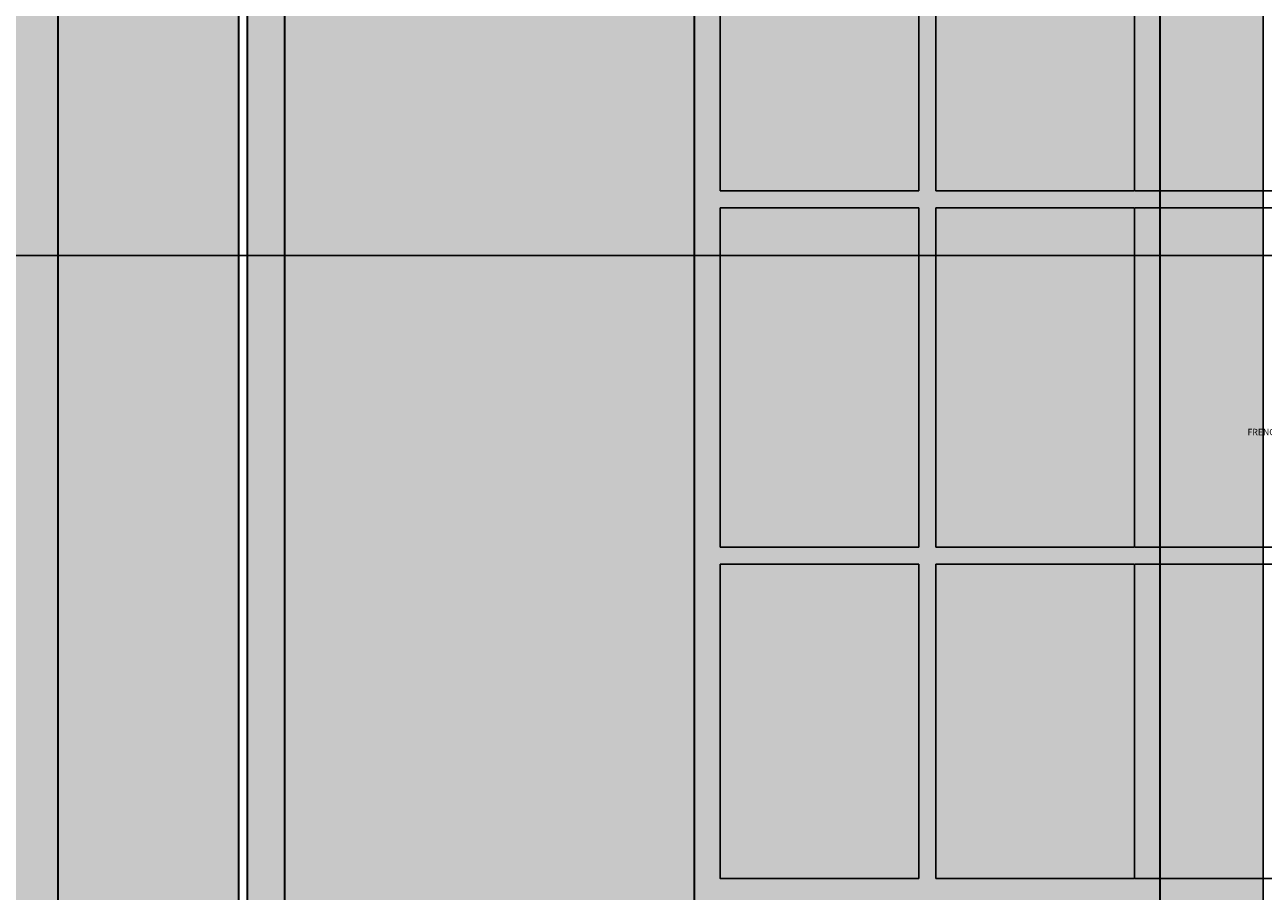
# Model space of a CAD drawing. Units: inches. Extents: x 62 to 566, y 66 to 528.
# Tile 4 of 20: x 138 to 284, y 162 to 264. Entities that reach past the tile are written whole.
import ezdxf

# ---------------------------------------------------------------- set-up
doc = ezdxf.new("R2010")
doc.units = ezdxf.units.IN
doc.header["$MEASUREMENT"] = 0
for name, color, linetype, lineweight in [('A-ANNO-DIMS', 2, 'Continuous', 18), ('A-ELEV', 7, 'Continuous', 35), ('A-GLAZ', 3, 'Continuous', 25), ('A-WALL-PATT', 8, 'Continuous', 13)]:
    doc.layers.add(name, color=color, linetype=linetype, lineweight=lineweight)
doc.styles.get("Standard").update_dxf_attribs({"font": 'arial.ttf'})
doc.dimstyles.get("Standard").update_dxf_attribs({"dimtxt": 0.75, "dimasz": 0.18, "dimexe": 0.18, "dimexo": 0.0625, "dimgap": 0.09, "dimtad": 0, "dimtih": 1, "dimtoh": 1, "dimdec": 4, "dimzin": 0, "dimdsep": 46, "dimlunit": 4, "dimtxsty": 'Standard', "dimcen": 0.09, "dimadec": 0, "dimazin": 0, "dimtfac": 1, "dimtdec": 4, "dimtofl": 0, "dimtmove": 0, "dimatfit": 3, "dimfxl": 1, "dimtolj": 1, "dimtzin": 0, "dimarcsym": 0})

# ---------------------------------------------------------------- blocks, each defined once
blk = doc.blocks.new('WIN-FRENCH-GRID')
for p, q in [((26.39, 108.06), (26.39, 83.9)), ((28.39, 108.06), (28.39, 83.9)), ((26.39, 83.9), (3, 83.9)), ((51.78, 83.9), (28.39, 83.9)), ((26.39, 81.9), (3, 81.9)), ((26.39, 81.9), (26.39, 41.97)), ((51.78, 81.9), (28.39, 81.9)), ((28.39, 81.9), (28.39, 41.97)), ((26.39, 41.97), (3, 41.97)), ((51.78, 41.97), (28.39, 41.97)), ((26.39, 39.97), (3, 39.97)), ((26.39, 39.97), (26.39, 3)), ((51.78, 39.97), (28.39, 39.97)), ((28.39, 39.97), (28.39, 3))]:
    blk.add_line(p, q)
blk.add_lwpolyline([(0, 111.06), (54.78, 111.06), (54.78, 0), (0, 0)], close=True)
for points in [[(3, 83.9), (3, 108.06), (26.39, 108.06)], [(28.39, 108.06), (51.78, 108.06), (51.78, 83.9)], [(3, 41.97), (3, 81.9)], [(51.78, 81.9), (51.78, 41.97)], [(26.39, 3), (3, 3), (3, 39.97)], [(51.78, 39.97), (51.78, 3), (28.39, 3)]]:
    blk.add_lwpolyline(points)
blk = doc.blocks.new('*D5')
at = {"layer": 'A-ANNO-DIMS', "color": 0, "lineweight": -2, "transparency": 16777216}
for p, q in [((272.12, 271.41), (288.9, 271.41)), ((288.72, 271.23), (288.72, 216.36)), ((288.72, 160.53), (288.72, 215.41)), ((272.12, 160.35), (288.9, 160.35))]:
    blk.add_line(p, q, dxfattribs=at)
at = {"layer": 'A-ANNO-DIMS', "color": 0, "transparency": 16777216}
for points in [[(288.69, 271.23), (288.75, 271.23), (288.72, 271.41)], [(288.69, 160.53), (288.75, 160.53), (288.72, 160.35)]]:
    blk.add_solid(points, dxfattribs=at)
at = {"layer": 'Defpoints', "color": 0, "transparency": 16777216}
for p in [(272.06, 271.41), (288.72, 271.41), (272.06, 160.35)]:
    blk.add_point(p, dxfattribs=at)
at = {"layer": 'A-ANNO-DIMS', "color": 0, "transparency": 16777216, "insert": (288.72, 215.88), "char_height": 0.75, "attachment_point": 5}
blk.add_mtext('\\A1;FRENCH WINDOW 111 TYP.', dxfattribs=at)
blk = doc.blocks.new('*D8')
at = {"layer": 'A-ANNO-DIMS', "color": 0, "lineweight": -2, "transparency": 16777216}
for p, q in [((284.2, 271.35), (284.2, 65.94)), ((125.94, 126.31), (125.94, 65.94)), ((126.12, 66.12), (203.46, 66.12)), ((284.02, 66.12), (206.68, 66.12))]:
    blk.add_line(p, q, dxfattribs=at)
at = {"layer": 'A-ANNO-DIMS', "color": 0, "transparency": 16777216}
for points in [[(126.12, 66.15), (126.12, 66.09), (125.94, 66.12)], [(284.02, 66.15), (284.02, 66.09), (284.2, 66.12)]]:
    blk.add_solid(points, dxfattribs=at)
at = {"layer": 'Defpoints', "color": 0, "transparency": 16777216}
for p in [(284.2, 271.41), (125.94, 126.37), (284.2, 66.12)]:
    blk.add_point(p, dxfattribs=at)
at = {"layer": 'A-ANNO-DIMS', "color": 0, "transparency": 16777216, "insert": (205.07, 66.12), "char_height": 0.75, "attachment_point": 5}
blk.add_mtext('\\A1;158.26', dxfattribs=at)
blk = doc.blocks.new('*D9')
at = {"layer": 'A-ANNO-DIMS', "color": 0, "lineweight": -2, "transparency": 16777216}
for p, q in [((284.2, 271.35), (284.2, 65.94)), ((316.21, 126.31), (316.21, 65.94)), ((284.38, 66.12), (298.92, 66.12)), ((316.03, 66.12), (301.49, 66.12))]:
    blk.add_line(p, q, dxfattribs=at)
at = {"layer": 'A-ANNO-DIMS', "color": 0, "transparency": 16777216}
for points in [[(284.38, 66.15), (284.38, 66.09), (284.2, 66.12)], [(316.03, 66.15), (316.03, 66.09), (316.21, 66.12)]]:
    blk.add_solid(points, dxfattribs=at)
at = {"layer": 'Defpoints', "color": 0, "transparency": 16777216}
for p in [(284.2, 271.41), (316.21, 126.37), (316.21, 66.12)]:
    blk.add_point(p, dxfattribs=at)
at = {"layer": 'A-ANNO-DIMS', "color": 0, "transparency": 16777216, "insert": (300.21, 66.12), "char_height": 0.75, "attachment_point": 5}
blk.add_mtext('\\A1;32.01', dxfattribs=at)
blk = doc.blocks.new('*D35')
at = {"layer": 'A-ANNO-DIMS', "color": 0, "lineweight": -2, "transparency": 16777216}
for p, q in [((125.94, 461.98), (125.94, 65.94)), ((142.39, 445.04), (142.39, 65.94)), ((126.12, 66.12), (132.55, 66.12)), ((142.21, 66.12), (135.77, 66.12))]:
    blk.add_line(p, q, dxfattribs=at)
at = {"layer": 'A-ANNO-DIMS', "color": 0, "transparency": 16777216}
for points in [[(126.12, 66.15), (126.12, 66.09), (125.94, 66.12)], [(142.21, 66.15), (142.21, 66.09), (142.39, 66.12)]]:
    blk.add_solid(points, dxfattribs=at)
at = {"layer": 'Defpoints', "color": 0, "transparency": 16777216}
for p in [(125.94, 462.04), (142.39, 445.11), (142.39, 66.12)]:
    blk.add_point(p, dxfattribs=at)
at = {"layer": 'A-ANNO-DIMS', "color": 0, "transparency": 16777216, "insert": (134.16, 66.12), "char_height": 0.75, "attachment_point": 5}
blk.add_mtext('\\A1;16.443', dxfattribs=at)
blk = doc.blocks.new('*D36')
at = {"layer": 'A-ANNO-DIMS', "color": 0, "lineweight": -2, "transparency": 16777216}
for p, q in [((142.39, 445.04), (142.39, 65.94)), ((163.65, 427.41), (163.65, 65.94)), ((142.57, 66.12), (151.66, 66.12)), ((163.47, 66.12), (154.38, 66.12))]:
    blk.add_line(p, q, dxfattribs=at)
at = {"layer": 'A-ANNO-DIMS', "color": 0, "transparency": 16777216}
for points in [[(142.57, 66.15), (142.57, 66.09), (142.39, 66.12)], [(163.47, 66.15), (163.47, 66.09), (163.65, 66.12)]]:
    blk.add_solid(points, dxfattribs=at)
at = {"layer": 'Defpoints', "color": 0, "transparency": 16777216}
for p in [(142.39, 445.11), (163.65, 427.48), (163.65, 66.12)]:
    blk.add_point(p, dxfattribs=at)
at = {"layer": 'A-ANNO-DIMS', "color": 0, "transparency": 16777216, "insert": (153.02, 66.12), "char_height": 0.75, "attachment_point": 5}
blk.add_mtext('\\A1;21.27', dxfattribs=at)
blk = doc.blocks.new('*D37')
at = {"layer": 'A-ANNO-DIMS', "color": 0, "lineweight": -2, "transparency": 16777216}
for p, q in [((163.65, 427.41), (163.65, 65.94)), ((169.04, 420.53), (169.04, 65.94)), ((163.83, 66.12), (164.99, 66.12)), ((168.86, 66.12), (167.71, 66.12))]:
    blk.add_line(p, q, dxfattribs=at)
at = {"layer": 'A-ANNO-DIMS', "color": 0, "transparency": 16777216}
for points in [[(163.83, 66.15), (163.83, 66.09), (163.65, 66.12)], [(168.86, 66.15), (168.86, 66.09), (169.04, 66.12)]]:
    blk.add_solid(points, dxfattribs=at)
at = {"layer": 'Defpoints', "color": 0, "transparency": 16777216}
for p in [(163.65, 427.48), (169.04, 420.6), (169.04, 66.12)]:
    blk.add_point(p, dxfattribs=at)
at = {"layer": 'A-ANNO-DIMS', "color": 0, "transparency": 16777216, "insert": (166.35, 66.12), "char_height": 0.75, "attachment_point": 5}
blk.add_mtext('\\A1;5.388', dxfattribs=at)
blk = doc.blocks.new('*D38')
at = {"layer": 'A-ANNO-DIMS', "color": 0, "lineweight": -2, "transparency": 16777216}
for p, q in [((169.04, 420.53), (169.04, 65.94)), ((217.28, 420.53), (217.28, 65.94)), ((169.22, 66.12), (191.79, 66.12)), ((217.1, 66.12), (194.53, 66.12))]:
    blk.add_line(p, q, dxfattribs=at)
at = {"layer": 'A-ANNO-DIMS', "color": 0, "transparency": 16777216}
for points in [[(169.22, 66.15), (169.22, 66.09), (169.04, 66.12)], [(217.1, 66.15), (217.1, 66.09), (217.28, 66.12)]]:
    blk.add_solid(points, dxfattribs=at)
at = {"layer": 'Defpoints', "color": 0, "transparency": 16777216}
for p in [(169.04, 420.6), (217.28, 420.6), (217.28, 66.12)]:
    blk.add_point(p, dxfattribs=at)
at = {"layer": 'A-ANNO-DIMS', "color": 0, "transparency": 16777216, "insert": (193.16, 66.12), "char_height": 0.75, "attachment_point": 5}
blk.add_mtext('\\A1;48.23', dxfattribs=at)
blk = doc.blocks.new('*D39')
at = {"layer": 'A-ANNO-DIMS', "color": 0, "lineweight": -2, "transparency": 16777216}
for p, q in [((284.2, 445.04), (284.2, 65.94)), ((217.28, 420.53), (217.28, 65.94)), ((217.46, 66.12), (249.38, 66.12)), ((284.02, 66.12), (252.1, 66.12))]:
    blk.add_line(p, q, dxfattribs=at)
at = {"layer": 'A-ANNO-DIMS', "color": 0, "transparency": 16777216}
for points in [[(217.46, 66.15), (217.46, 66.09), (217.28, 66.12)], [(284.02, 66.15), (284.02, 66.09), (284.2, 66.12)]]:
    blk.add_solid(points, dxfattribs=at)
at = {"layer": 'Defpoints', "color": 0, "transparency": 16777216}
for p in [(284.2, 445.11), (217.28, 420.6), (284.2, 66.12)]:
    blk.add_point(p, dxfattribs=at)
at = {"layer": 'A-ANNO-DIMS', "color": 0, "transparency": 16777216, "insert": (250.74, 66.12), "char_height": 0.75, "attachment_point": 5}
blk.add_mtext('\\A1;66.93', dxfattribs=at)
blk = doc.blocks.new('*D40')
at = {"layer": 'A-ANNO-DIMS', "color": 0, "lineweight": -2, "transparency": 16777216}
for p, q in [((284.2, 445.04), (284.2, 65.94)), ((316.21, 417.64), (316.21, 65.94)), ((284.38, 66.12), (298.92, 66.12)), ((316.03, 66.12), (301.49, 66.12))]:
    blk.add_line(p, q, dxfattribs=at)
at = {"layer": 'A-ANNO-DIMS', "color": 0, "transparency": 16777216}
for points in [[(284.38, 66.15), (284.38, 66.09), (284.2, 66.12)], [(316.03, 66.15), (316.03, 66.09), (316.21, 66.12)]]:
    blk.add_solid(points, dxfattribs=at)
at = {"layer": 'Defpoints', "color": 0, "transparency": 16777216}
for p in [(284.2, 445.11), (316.21, 417.71), (316.21, 66.12)]:
    blk.add_point(p, dxfattribs=at)
at = {"layer": 'A-ANNO-DIMS', "color": 0, "transparency": 16777216, "insert": (300.21, 66.12), "char_height": 0.75, "attachment_point": 5}
blk.add_mtext('\\A1;32.01', dxfattribs=at)
blk = doc.blocks.new('*D73')
at = {"layer": 'A-ANNO-DIMS', "color": 0, "lineweight": -2, "transparency": 16777216}
for p, q in [((316.15, 236.66), (63.47, 236.66)), ((63.65, 236.48), (63.65, 181.99)), ((63.65, 126.55), (63.65, 181.04)), ((316.15, 126.37), (63.47, 126.37))]:
    blk.add_line(p, q, dxfattribs=at)
at = {"layer": 'A-ANNO-DIMS', "color": 0, "transparency": 16777216}
for points in [[(63.62, 236.48), (63.68, 236.48), (63.65, 236.66)], [(63.62, 126.55), (63.68, 126.55), (63.65, 126.37)]]:
    blk.add_solid(points, dxfattribs=at)
at = {"layer": 'Defpoints', "color": 0, "transparency": 16777216}
for p in [(63.65, 236.66), (316.21, 236.66), (316.21, 126.37)]:
    blk.add_point(p, dxfattribs=at)
at = {"layer": 'A-ANNO-DIMS', "color": 0, "transparency": 16777216, "insert": (63.65, 181.52), "char_height": 0.75, "attachment_point": 5}
blk.add_mtext('\\A1;110.3', dxfattribs=at)
blk = doc.blocks.new('*D82')
at = {"layer": 'A-ANNO-DIMS', "color": 0, "lineweight": -2, "transparency": 16777216}
for p, q in [((296.38, 279.98), (296.38, 65.94)), ((284.2, 271.35), (284.2, 65.94)), ((284.38, 66.12), (288.68, 66.12)), ((296.2, 66.12), (291.9, 66.12))]:
    blk.add_line(p, q, dxfattribs=at)
at = {"layer": 'A-ANNO-DIMS', "color": 0, "transparency": 16777216}
for points in [[(284.38, 66.15), (284.38, 66.09), (284.2, 66.12)], [(296.2, 66.15), (296.2, 66.09), (296.38, 66.12)]]:
    blk.add_solid(points, dxfattribs=at)
at = {"layer": 'Defpoints', "color": 0, "transparency": 16777216}
for p in [(296.38, 280.04), (284.2, 271.41), (296.38, 66.12)]:
    blk.add_point(p, dxfattribs=at)
at = {"layer": 'A-ANNO-DIMS', "color": 0, "transparency": 16777216, "insert": (290.29, 66.12), "char_height": 0.75, "attachment_point": 5}
blk.add_mtext('\\A1;12.173', dxfattribs=at)
blk = doc.blocks.new('*D122')
at = {"layer": 'A-ANNO-DIMS', "color": 0, "lineweight": -2, "transparency": 16777216}
for p, q in [((269.12, 163.35), (564.47, 163.35)), ((564.29, 163.17), (564.29, 162.33)), ((272.12, 160.35), (564.47, 160.35)), ((564.29, 160.53), (564.29, 161.38))]:
    blk.add_line(p, q, dxfattribs=at)
at = {"layer": 'A-ANNO-DIMS', "color": 0, "transparency": 16777216}
for points in [[(564.26, 163.17), (564.32, 163.17), (564.29, 163.35)], [(564.26, 160.53), (564.32, 160.53), (564.29, 160.35)]]:
    blk.add_solid(points, dxfattribs=at)
at = {"layer": 'Defpoints', "color": 0, "transparency": 16777216}
for p in [(269.06, 163.35), (564.29, 163.35), (272.06, 160.35)]:
    blk.add_point(p, dxfattribs=at)
at = {"layer": 'A-ANNO-DIMS', "color": 0, "transparency": 16777216, "insert": (564.29, 161.85), "char_height": 0.75, "attachment_point": 5}
blk.add_mtext('\\A1;3', dxfattribs=at)
blk = doc.blocks.new('*D123')
at = {"layer": 'A-ANNO-DIMS', "color": 0, "lineweight": -2, "transparency": 16777216}
for p, q in [((269.12, 200.32), (564.47, 200.32)), ((564.29, 200.14), (564.29, 182.31)), ((564.29, 163.53), (564.29, 181.37)), ((269.12, 163.35), (564.47, 163.35))]:
    blk.add_line(p, q, dxfattribs=at)
at = {"layer": 'A-ANNO-DIMS', "color": 0, "transparency": 16777216}
for points in [[(564.26, 200.14), (564.32, 200.14), (564.29, 200.32)], [(564.26, 163.53), (564.32, 163.53), (564.29, 163.35)]]:
    blk.add_solid(points, dxfattribs=at)
at = {"layer": 'Defpoints', "color": 0, "transparency": 16777216}
for p in [(269.06, 200.32), (564.29, 200.32), (269.06, 163.35)]:
    blk.add_point(p, dxfattribs=at)
at = {"layer": 'A-ANNO-DIMS', "color": 0, "transparency": 16777216, "insert": (564.29, 181.84), "char_height": 0.75, "attachment_point": 5}
blk.add_mtext('\\A1;36.97', dxfattribs=at)
blk = doc.blocks.new('*D124')
at = {"layer": 'A-ANNO-DIMS', "color": 0, "lineweight": -2, "transparency": 16777216}
for p, q in [((269.12, 202.32), (564.47, 202.32)), ((564.29, 202.14), (564.29, 201.79)), ((269.12, 200.32), (564.47, 200.32)), ((564.29, 200.5), (564.29, 200.86))]:
    blk.add_line(p, q, dxfattribs=at)
at = {"layer": 'A-ANNO-DIMS', "color": 0, "transparency": 16777216}
for points in [[(564.26, 202.14), (564.32, 202.14), (564.29, 202.32)], [(564.26, 200.5), (564.32, 200.5), (564.29, 200.32)]]:
    blk.add_solid(points, dxfattribs=at)
at = {"layer": 'Defpoints', "color": 0, "transparency": 16777216}
for p in [(269.06, 202.32), (564.29, 202.32), (269.06, 200.32)]:
    blk.add_point(p, dxfattribs=at)
at = {"layer": 'A-ANNO-DIMS', "color": 0, "transparency": 16777216, "insert": (564.29, 201.32), "char_height": 0.75, "attachment_point": 5}
blk.add_mtext('\\A1;2', dxfattribs=at)
blk = doc.blocks.new('*D125')
at = {"layer": 'A-ANNO-DIMS', "color": 0, "lineweight": -2, "transparency": 16777216}
for p, q in [((269.12, 242.25), (564.47, 242.25)), ((564.29, 242.07), (564.29, 222.76)), ((564.29, 202.5), (564.29, 221.81)), ((269.12, 202.32), (564.47, 202.32))]:
    blk.add_line(p, q, dxfattribs=at)
at = {"layer": 'A-ANNO-DIMS', "color": 0, "transparency": 16777216}
for points in [[(564.26, 242.07), (564.32, 242.07), (564.29, 242.25)], [(564.26, 202.5), (564.32, 202.5), (564.29, 202.32)]]:
    blk.add_solid(points, dxfattribs=at)
at = {"layer": 'Defpoints', "color": 0, "transparency": 16777216}
for p in [(269.06, 242.25), (564.29, 242.25), (269.06, 202.32)]:
    blk.add_point(p, dxfattribs=at)
at = {"layer": 'A-ANNO-DIMS', "color": 0, "transparency": 16777216, "insert": (564.29, 222.29), "char_height": 0.75, "attachment_point": 5}
blk.add_mtext('\\A1;39.93', dxfattribs=at)
blk = doc.blocks.new('*D126')
at = {"layer": 'A-ANNO-DIMS', "color": 0, "lineweight": -2, "transparency": 16777216}
for p, q in [((269.12, 244.25), (564.47, 244.25)), ((564.29, 244.07), (564.29, 243.72)), ((269.12, 242.25), (564.47, 242.25)), ((564.29, 242.43), (564.29, 242.78))]:
    blk.add_line(p, q, dxfattribs=at)
at = {"layer": 'A-ANNO-DIMS', "color": 0, "transparency": 16777216}
for points in [[(564.26, 244.07), (564.32, 244.07), (564.29, 244.25)], [(564.26, 242.43), (564.32, 242.43), (564.29, 242.25)]]:
    blk.add_solid(points, dxfattribs=at)
at = {"layer": 'Defpoints', "color": 0, "transparency": 16777216}
for p in [(269.06, 244.25), (564.29, 244.25), (269.06, 242.25)]:
    blk.add_point(p, dxfattribs=at)
at = {"layer": 'A-ANNO-DIMS', "color": 0, "transparency": 16777216, "insert": (564.29, 243.25), "char_height": 0.75, "attachment_point": 5}
blk.add_mtext('\\A1;2', dxfattribs=at)
blk = doc.blocks.new('*D127')
at = {"layer": 'A-ANNO-DIMS', "color": 0, "lineweight": -2, "transparency": 16777216}
for p, q in [((269.12, 268.41), (564.47, 268.41)), ((564.29, 268.23), (564.29, 256.8)), ((564.29, 244.43), (564.29, 255.86)), ((269.12, 244.25), (564.47, 244.25))]:
    blk.add_line(p, q, dxfattribs=at)
at = {"layer": 'A-ANNO-DIMS', "color": 0, "transparency": 16777216}
for points in [[(564.26, 268.23), (564.32, 268.23), (564.29, 268.41)], [(564.26, 244.43), (564.32, 244.43), (564.29, 244.25)]]:
    blk.add_solid(points, dxfattribs=at)
at = {"layer": 'Defpoints', "color": 0, "transparency": 16777216}
for p in [(269.06, 268.41), (564.29, 268.41), (269.06, 244.25)]:
    blk.add_point(p, dxfattribs=at)
at = {"layer": 'A-ANNO-DIMS', "color": 0, "transparency": 16777216, "insert": (564.29, 256.33), "char_height": 0.75, "attachment_point": 5}
blk.add_mtext('\\A1;24.16', dxfattribs=at)

msp = doc.modelspace()

# ---------------------------------------------------------------- hatches: boundary and pattern name
at = {"layer": 'A-WALL-PATT'}
h = msp.add_hatch(color=256, dxfattribs=at)
h.dxf.hatch_style = 1
h.paths.add_polyline_path([(416.0836, 462.0423), (125.9418, 462.0423), (125.9418, 414.3686), (125.9418, 270.3686), (125.9418, 126.3686), (142.3851, 126.3686), (142.3851, 270.3686), (142.3851, 414.3686), (142.3851, 445.1064), (284.2021, 445.1064), (416.0836, 445.1064)])
h.paths.add_polyline_path([(435.3945, 503.0423), (426.3652, 503.0423), (120.4058, 503.0423), (120.4058, 501.0423), (125.9418, 501.0423), (416.0836, 501.0423), (426.3652, 501.0423), (430.6938, 501.0423), (435.3945, 501.0423)])
h.paths.add_polyline_path([(439.6878, 352.4848), (392.4793, 352.4848), (392.4793, 307.4128), (217.2752, 307.4128), (217.2752, 295.4098), (217.2752, 271.4128), (272.0586, 271.4128), (439.6878, 271.4128)])
h.paths.add_polyline_path([(248.0143, 297.1682), (255.6783, 297.1682), (255.6783, 280.0423), (248.0143, 280.0423)], flags=16)
h.paths.add_polyline_path([(235.4641, 280.0423), (227.8001, 280.0423), (227.8001, 297.1682), (235.4641, 297.1682)], flags=16)
h.paths.add_polyline_path([(270.4427, 297.1682), (278.1067, 297.1682), (278.1067, 280.0423), (270.4427, 280.0423)], flags=16)
h.paths.add_polyline_path([(296.3755, 297.1682), (304.0395, 297.1682), (304.0395, 280.0423), (296.3755, 280.0423)], flags=16)
h.paths.add_polyline_path([(319.2543, 297.1682), (326.9183, 297.1682), (326.9183, 280.0423), (319.2543, 280.0423)], flags=16)
h.paths.add_polyline_path([(341.2622, 297.1682), (348.9262, 297.1682), (348.9262, 280.0423), (341.2622, 280.0423)], flags=16)
h.paths.add_polyline_path([(389.2857, 298.3985), (433.8102, 298.3985), (433.8102, 294.9497), (389.2857, 294.9497)], flags=16)
h.paths.add_polyline_path([(389.2857, 291.6038), (433.8102, 291.6038), (433.8102, 288.155), (389.2857, 288.155)], flags=16)
h.paths.add_polyline_path([(389.2857, 284.9607), (433.8102, 284.9607), (433.8102, 281.5119), (389.2857, 281.5119)], flags=16)
h.paths.add_polyline_path([(403.5849, 311.4736), (403.5849, 317.4388), (433.1636, 317.4388), (433.1636, 311.4736)], flags=16)
h.paths.add_polyline_path([(403.5849, 323.1329), (403.5849, 329.0982), (433.1636, 329.0982), (433.1636, 323.1329)], flags=16)
h.paths.add_polyline_path([(403.5849, 334.5211), (403.5849, 340.4863), (433.1636, 340.4863), (433.1636, 334.5211)], flags=16)
h.paths.add_polyline_path([(272.0586, 160.3545), (217.2752, 160.3545), (217.2752, 129.0504), (217.2752, 126.3686), (272.0586, 126.3686)], flags=17)
h.paths.add_polyline_path([(220.5897, 149.5749), (220.5897, 152.296), (267.7931, 152.296), (267.7931, 149.5749)], flags=16)
h.paths.add_polyline_path([(267.7931, 146.6724), (267.7931, 143.9513), (220.5897, 143.9513), (220.5897, 146.6724)], flags=16)
h.paths.add_polyline_path([(220.5897, 155.3799), (220.5897, 158.101), (267.7931, 158.101), (267.7931, 155.3799)], flags=16)
h.paths.add_polyline_path([(267.7931, 140.686), (267.7931, 137.9649), (220.5897, 137.9649), (220.5897, 140.686)], flags=16)
h.paths.add_polyline_path([(267.7931, 135.516), (267.7931, 132.7949), (220.5897, 132.7949), (220.5897, 135.516)], flags=16)
h = msp.add_hatch(dxfattribs=at)
h.set_pattern_fill('ANSI36', color=256, scale=8.8)
h.paths.add_polyline_path([(217.2752, 420.597), (169.0431, 420.597), (169.0431, 126.3686), (217.2752, 126.3686), (217.2752, 129.0504), (217.2752, 271.4128), (217.2752, 295.4128), (217.2752, 307.4128)])
h.paths.add_polyline_path([(282.3509, 501.0423), (125.9418, 501.0423), (125.9418, 465.0423), (282.3509, 465.0423)])
h.paths.add_polyline_path([(209.709, 476.6506), (202.045, 476.6506), (202.045, 493.7764), (209.709, 493.7764)], flags=16)
h.paths.add_polyline_path([(193.9913, 476.6506), (186.3273, 476.6506), (186.3273, 493.7764), (193.9913, 493.7764)], flags=16)
h.paths.add_polyline_path([(177.9243, 476.6506), (170.2603, 476.6506), (170.2603, 493.7764), (177.9243, 493.7764)], flags=16)
h.paths.add_polyline_path([(163.2545, 476.3015), (155.5905, 476.3015), (155.5905, 493.4274), (163.2545, 493.4274)], flags=16)
h.paths.add_polyline_path([(148.2354, 476.3015), (140.5713, 476.3015), (140.5713, 493.4274), (148.2354, 493.4274)], flags=16)
h.paths.add_polyline_path([(284.2021, 126.3686), (87.8962, 126.3686), (87.8962, 114.3686), (87.8962, 90.3686), (284.2021, 90.3686)])
h.paths.add_polyline_path([(474.1214, 126.3686), (396.433, 126.3686), (396.433, 90.3686), (474.1214, 90.3686)])
h = msp.add_hatch(color=256, dxfattribs=at)
h.dxf.hatch_style = 1
h.paths.add_polyline_path([(416.0836, 501.0423), (282.3509, 501.0423), (282.3509, 465.0423), (416.0836, 465.0423)])
h.paths.add_polyline_path([(284.2021, 420.597), (272.0586, 420.597), (272.0586, 309.5388), (272.0586, 307.4128), (284.2021, 307.4128)], flags=17)
h.paths.add_polyline_path([(284.2021, 445.1064), (142.3851, 445.1064), (142.3851, 414.3686), (142.3851, 270.3686), (142.3851, 126.3686), (163.6548, 126.3686), (163.6548, 270.5016), (163.6548, 414.5016), (163.6548, 427.4752), (284.2021, 427.4752)])
h.paths.add_polyline_path([(235.4641, 297.1682), (227.8001, 297.1682), (227.8001, 280.0423), (235.4641, 280.0423)], flags=17)
h.paths.add_polyline_path([(255.6783, 297.1682), (248.0143, 297.1682), (248.0143, 280.0423), (255.6783, 280.0423)], flags=17)
h.paths.add_polyline_path([(278.1067, 297.1682), (270.4427, 297.1682), (270.4427, 280.0423), (278.1067, 280.0423)], flags=17)
h.paths.add_polyline_path([(304.0395, 297.1682), (296.3755, 297.1682), (296.3755, 280.0423), (304.0395, 280.0423)])
h.paths.add_polyline_path([(326.9183, 297.1682), (319.2543, 297.1682), (319.2543, 280.0423), (326.9183, 280.0423)])
h.paths.add_polyline_path([(348.9262, 297.1682), (341.2622, 297.1682), (341.2622, 280.0423), (348.9262, 280.0423)])
h.paths.add_polyline_path([(433.8102, 284.9607), (389.2857, 284.9607), (389.2857, 281.5119), (433.8102, 281.5119)])
h.paths.add_polyline_path([(433.8102, 291.6038), (389.2857, 291.6038), (389.2857, 288.155), (433.8102, 288.155)])
h.paths.add_polyline_path([(433.8102, 298.3985), (389.2857, 298.3985), (389.2857, 294.9497), (433.8102, 294.9497)])
h.paths.add_polyline_path([(433.1636, 317.4388), (403.5849, 317.4388), (403.5849, 311.4736), (433.1636, 311.4736)])
h.paths.add_polyline_path([(433.1636, 329.0982), (403.5849, 329.0982), (403.5849, 323.1329), (433.1636, 323.1329)])
h.paths.add_polyline_path([(433.1636, 340.4863), (403.5849, 340.4863), (403.5849, 334.5211), (433.1636, 334.5211)])
h.paths.add_polyline_path([(284.2021, 271.4128), (272.0586, 271.4128), (272.0586, 160.3545), (272.0586, 126.3686), (284.2021, 126.3686)])
h.paths.add_polyline_path([(267.7931, 158.101), (220.5897, 158.101), (220.5897, 155.3799), (267.7931, 155.3799)], flags=17)
h.paths.add_polyline_path([(267.7931, 152.296), (220.5897, 152.296), (220.5897, 149.5749), (267.7931, 149.5749)], flags=17)
h.paths.add_polyline_path([(267.7931, 146.6724), (220.5897, 146.6724), (220.5897, 143.9513), (267.7931, 143.9513)], flags=17)
h.paths.add_polyline_path([(267.7931, 140.686), (220.5897, 140.686), (220.5897, 137.9649), (267.7931, 137.9649)], flags=17)
h.paths.add_polyline_path([(267.7931, 135.516), (220.5897, 135.516), (220.5897, 132.7949), (267.7931, 132.7949)], flags=17)
h.paths.add_polyline_path([(148.2354, 493.4274), (140.5713, 493.4274), (140.5713, 476.3015), (148.2354, 476.3015)])
h.paths.add_polyline_path([(163.2545, 493.4274), (155.5905, 493.4274), (155.5905, 476.3015), (163.2545, 476.3015)])
h.paths.add_polyline_path([(177.9243, 493.7764), (170.2603, 493.7764), (170.2603, 476.6506), (177.9243, 476.6506)])
h.paths.add_polyline_path([(193.9913, 493.7764), (186.3273, 493.7764), (186.3273, 476.6506), (193.9913, 476.6506)])
h.paths.add_polyline_path([(209.709, 493.7764), (202.045, 493.7764), (202.045, 476.6506), (209.709, 476.6506)])
h = msp.add_hatch(color=256, dxfattribs=at)
h.dxf.hatch_style = 1
h.paths.add_polyline_path([(430.6938, 462.0423), (416.0836, 462.0423), (416.0836, 445.1064), (430.6938, 445.1064)])
h.paths.add_polyline_path([(169.0431, 420.597), (284.2021, 420.597), (284.2021, 426.4752), (164.6548, 426.4752), (164.6548, 414.5016), (164.6548, 126.3686), (169.0431, 126.3686)])
h = msp.add_hatch(color=256, dxfattribs=at)
h.dxf.hatch_style = 1
h.paths.add_polyline_path([(272.0586, 420.597), (217.2752, 420.597), (217.2752, 309.5388), (272.0586, 309.5388)])
h.paths.add_polyline_path([(245.6669, 393.435), (245.6669, 417.597), (269.0586, 417.597), (269.0586, 393.435)], flags=16)
h.paths.add_polyline_path([(245.6669, 391.435), (269.0586, 391.435), (269.0586, 351.5079), (245.6669, 351.5079)], flags=16)
h.paths.add_polyline_path([(243.6669, 393.435), (220.2752, 393.435), (220.2752, 417.597), (243.6669, 417.597)], flags=16)
h.paths.add_polyline_path([(243.6669, 391.435), (243.6669, 351.5079), (220.2752, 351.5079), (220.2752, 391.435)], flags=16)
h.paths.add_polyline_path([(245.6669, 349.5079), (269.0586, 349.5079), (269.0586, 312.5388), (245.6669, 312.5388)], flags=16)
h.paths.add_polyline_path([(243.6669, 349.5079), (243.6669, 312.5388), (220.2752, 312.5388), (220.2752, 349.5079)], flags=16)
h.paths.add_polyline_path([(272.0586, 271.4128), (217.2752, 271.4128), (217.2752, 160.3545), (272.0586, 160.3545)])
h.paths.add_polyline_path([(243.6669, 268.4128), (243.6669, 244.2507), (220.2752, 244.2507), (220.2752, 268.4128)], flags=16)
h.paths.add_polyline_path([(245.6669, 268.4128), (269.0586, 268.4128), (269.0586, 244.2507), (245.6669, 244.2507)], flags=16)
h.paths.add_polyline_path([(243.6669, 242.2507), (243.6669, 202.3236), (220.2752, 202.3236), (220.2752, 242.2507)], flags=16)
h.paths.add_polyline_path([(245.6669, 242.2507), (269.0586, 242.2507), (269.0586, 202.3236), (245.6669, 202.3236)], flags=16)
h.paths.add_polyline_path([(243.6669, 200.3236), (243.6669, 163.3545), (220.2752, 163.3545), (220.2752, 200.3236)], flags=16)
h.paths.add_polyline_path([(245.6669, 200.3236), (269.0586, 200.3236), (269.0586, 163.3545), (245.6669, 163.3545)], flags=16)
h.paths.add_polyline_path([(272.0586, 309.5388), (217.2752, 309.5388), (217.2752, 307.4128), (272.0586, 307.4128)])
h = msp.add_hatch(color=256, dxfattribs=at)
h.dxf.hatch_style = 1
h.set_gradient(color1=(0, 0, 255), color2=(0, 0, 0))
h.paths.add_polyline_path([(243.6669, 417.597), (220.2752, 417.597), (220.2752, 393.435), (243.6669, 393.435)])
h.paths.add_polyline_path([(269.0586, 417.597), (245.6669, 417.597), (245.6669, 393.435), (269.0586, 393.435)])
h.paths.add_polyline_path([(269.0586, 391.435), (245.6669, 391.435), (245.6669, 351.5079), (269.0586, 351.5079)])
h.paths.add_polyline_path([(243.6669, 391.435), (220.2752, 391.435), (220.2752, 351.5079), (243.6669, 351.5079)])
h.paths.add_polyline_path([(243.6669, 349.5079), (220.2752, 349.5079), (220.2752, 312.5388), (243.6669, 312.5388)])
h.paths.add_polyline_path([(269.0586, 349.5079), (245.6669, 349.5079), (245.6669, 312.5388), (269.0586, 312.5388)])
h.paths.add_polyline_path([(243.6669, 268.4128), (220.2752, 268.4128), (220.2752, 244.2507), (243.6669, 244.2507)])
h.paths.add_polyline_path([(269.0586, 268.4128), (245.6669, 268.4128), (245.6669, 244.2507), (269.0586, 244.2507)])
h.paths.add_polyline_path([(269.0586, 242.2507), (245.6669, 242.2507), (245.6669, 202.3236), (269.0586, 202.3236)])
h.paths.add_polyline_path([(243.6669, 242.2507), (220.2752, 242.2507), (220.2752, 202.3236), (243.6669, 202.3236)])
h.paths.add_polyline_path([(243.6669, 200.3236), (220.2752, 200.3236), (220.2752, 163.3545), (243.6669, 163.3545)])
h.paths.add_polyline_path([(269.0586, 200.3236), (245.6669, 200.3236), (245.6669, 163.3545), (269.0586, 163.3545)])

# ---------------------------------------------------------------- linework, layer by layer
at = {"layer": 'A-ELEV'}
for p, q in [((169.0431, 126.3686), (169.0431, 420.597)), ((217.2752, 129.0504), (217.2752, 271.4128)), ((272.0586, 126.3686), (272.0586, 271.4128)), ((142.3851, 126.3686), (142.3851, 270.3686))]:
    msp.add_line(p, q, dxfattribs=at)
for points in [[(163.6548, 126.3686), (163.6548, 414.5016), (163.6548, 427.4752), (284.2021, 427.4752)], [(164.6548, 126.3686), (164.6548, 414.5016), (164.6548, 426.4752), (284.2021, 426.4752)]]:
    msp.add_lwpolyline(points, dxfattribs=at)

# ---------------------------------------------------------------- block references
at = {"layer": 'A-GLAZ'}
msp.add_blockref('WIN-FRENCH-GRID', (217.2752, 160.3545), dxfattribs=at)

# ---------------------------------------------------------------- dimensions: what is measured, and where the dimension line sits
at = {"layer": 'A-ANNO-DIMS'}
for base, p1, p2, override, picture, middle in [((142.3851, 66.1186), (125.9418, 462.0423), (142.3851, 445.1064), {"dimdec": 3, "dimlfac": 1, "dimrnd": 0, "dimzin": 0, "dimdsep": 46, "dimlunit": 2}, '*D35', (134.1634, 66.1186)), ((163.6548, 66.1186), (142.3851, 445.1064), (163.6548, 427.4752), {"dimdec": 2, "dimlfac": 1, "dimrnd": 0, "dimzin": 0, "dimdsep": 46, "dimlunit": 2}, '*D36', (153.0199, 66.1186)), ((284.2021, 66.1186), (217.2752, 420.597), (284.2021, 445.1064), {"dimdec": 2, "dimlfac": 1, "dimrnd": 0, "dimzin": 0, "dimdsep": 46, "dimlunit": 2}, '*D39', (250.7386, 66.1186)), ((316.2101, 66.1186), (284.2021, 445.1064), (316.2101, 417.7059), {"dimdec": 2, "dimlfac": 1, "dimrnd": 0, "dimzin": 0, "dimdsep": 46, "dimlunit": 2}, '*D40', (300.2061, 66.1186)), ((169.0431, 66.1186), (163.6548, 427.4752), (169.0431, 420.597), {"dimdec": 3, "dimlfac": 1, "dimrnd": 0, "dimzin": 0, "dimdsep": 46, "dimlunit": 2}, '*D37', (166.349, 66.1186)), ((217.2752, 66.1186), (169.0431, 420.597), (217.2752, 420.597), {"dimdec": 2, "dimlfac": 1, "dimrnd": 0, "dimzin": 0, "dimdsep": 46, "dimlunit": 2}, '*D38', (193.1592, 66.1186)), ((296.3755, 66.1186), (284.2021, 271.4128), (296.3755, 280.0423), {"dimdec": 3, "dimlfac": 1, "dimrnd": 0, "dimzin": 0, "dimdsep": 46, "dimlunit": 2}, '*D82', (290.2888, 66.1186)), ((284.2021, 66.1186), (125.9418, 126.3686), (284.2021, 271.4128), {"dimdec": 2, "dimlfac": 1, "dimrnd": 0, "dimzin": 0, "dimdsep": 46, "dimlunit": 2}, '*D8', (205.0719, 66.1186)), ((316.2101, 66.1186), (284.2021, 271.4128), (316.2101, 126.3686), {"dimdec": 2, "dimlfac": 1, "dimrnd": 0, "dimzin": 0, "dimdsep": 46, "dimlunit": 2}, '*D9', (300.2061, 66.1186))]:
    dim = msp.add_linear_dim(base=base, p1=p1, p2=p2, dimstyle='Standard', override=override, dxfattribs=at)
    dim.commit()
    dim.dimension.update_dxf_attribs({"geometry": picture, "text_midpoint": middle})
dim = msp.add_linear_dim(base=(288.7173, 271.4128), p1=(272.0586, 160.3545), p2=(272.0586, 271.4128), angle=90, text='FRENCH WINDOW <> TYP.', dimstyle='Standard', override={"dimdec": 0, "dimlfac": 1, "dimrnd": 0, "dimzin": 0, "dimdsep": 46, "dimlunit": 2}, dxfattribs=at)
dim.commit()
dim.dimension.update_dxf_attribs({"geometry": '*D5', "text_midpoint": (288.7173, 215.8836)})
for base, p1, p2, override, picture, middle in [((564.2868, 268.4128), (269.0586, 244.2507), (269.0586, 268.4128), {"dimdec": 2, "dimlfac": 1, "dimrnd": 0, "dimzin": 0, "dimdsep": 46, "dimlunit": 2}, '*D127', (564.2868, 256.3317)), ((564.2868, 244.2507), (269.0586, 242.2507), (269.0586, 244.2507), {"dimdec": 0, "dimlfac": 1, "dimrnd": 0, "dimzin": 0, "dimdsep": 46, "dimlunit": 2}, '*D126', (564.2868, 243.2507)), ((564.2868, 242.2507), (269.0586, 202.3236), (269.0586, 242.2507), {"dimdec": 2, "dimlfac": 1, "dimrnd": 0, "dimzin": 0, "dimdsep": 46, "dimlunit": 2}, '*D125', (564.2868, 222.2872)), ((63.6462, 236.6618), (316.2101, 126.3686), (316.2101, 236.6618), {"dimdec": 1, "dimlfac": 1, "dimrnd": 0, "dimzin": 0, "dimdsep": 46, "dimlunit": 2}, '*D73', (63.6462, 181.5152)), ((564.2868, 202.3236), (269.0586, 200.3236), (269.0586, 202.3236), {"dimdec": 0, "dimlfac": 1, "dimrnd": 0, "dimzin": 0, "dimdsep": 46, "dimlunit": 2}, '*D124', (564.2868, 201.3236)), ((564.2868, 200.3236), (269.0586, 163.3545), (269.0586, 200.3236), {"dimdec": 2, "dimlfac": 1, "dimrnd": 0, "dimzin": 0, "dimdsep": 46, "dimlunit": 2}, '*D123', (564.2868, 181.8391)), ((564.2868, 163.3545), (272.0586, 160.3545), (269.0586, 163.3545), {"dimdec": 0, "dimlfac": 1, "dimrnd": 0, "dimzin": 0, "dimdsep": 46, "dimlunit": 2}, '*D122', (564.2868, 161.8545))]:
    dim = msp.add_linear_dim(base=base, p1=p1, p2=p2, angle=90, dimstyle='Standard', override=override, dxfattribs=at)
    dim.commit()
    dim.dimension.update_dxf_attribs({"geometry": picture, "text_midpoint": middle})

doc.saveas('drawing.dxf')
